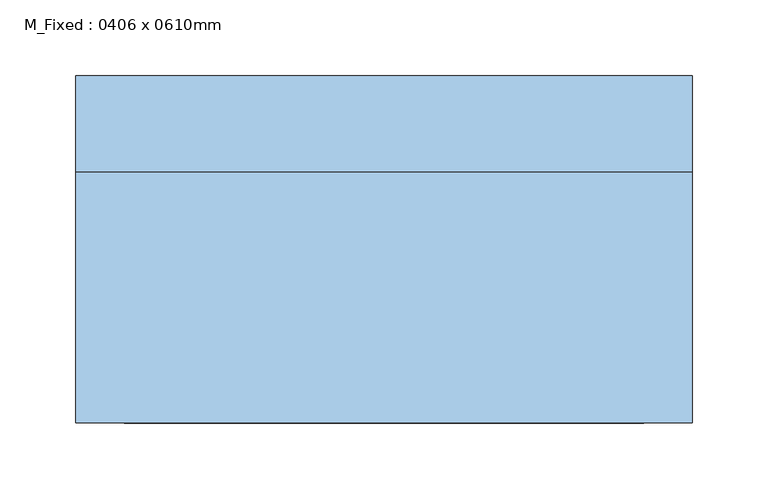
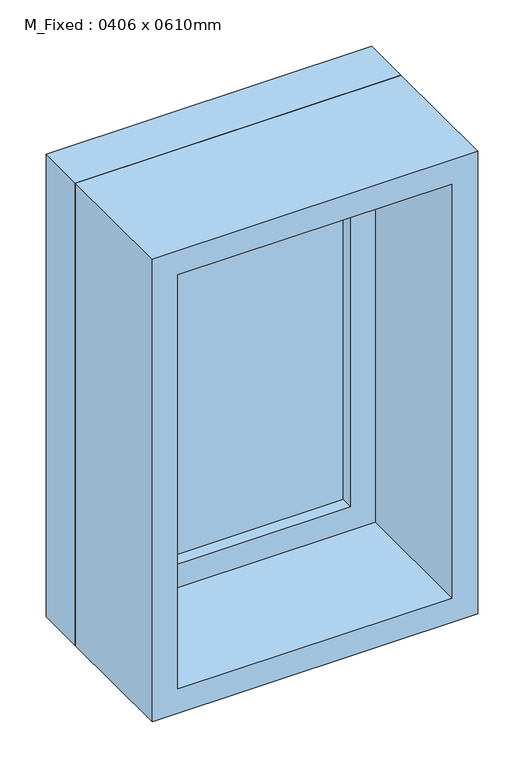
"""IFC4 building model written with IfcOpenShell, lengths in millimetres: window geometry, M_Fixed : 0406 x 0610mm."""

from ifc_helpers import new_model, si_unit, frame, origin, place, context, project, spatial, polyline, outline, extrude, source, transform, mapped, element, save


def m_fixed_0406_x_0610mm_6289636b(model_context):
    return source(origin(), model_context, "Body", "SweptSolid", [
        extrude(outline(polyline([(-140.0, 92.3), (140.0, 92.3), (140.0, 80.3), (-140.0, 80.3), (-140.0, 92.3)])), frame((0.0, 0.0, 978.0), z_axis=(0.0, 0.0, 1.0), x_axis=(1.0, 0.0, 0.0)), (0.0, 0.0, 1.0), 484.0),
        extrude(outline(polyline([(1506.0, -184.0), (934.0, -184.0), (934.0, 184.0), (1506.0, 184.0), (1506.0, -184.0)]), holes=[polyline([(1462.0, -140.0), (1462.0, 140.0), (978.0, 140.0), (978.0, -140.0), (1462.0, -140.0)])]), frame((0.0, 64.3, 0.0), z_axis=(0.0, 1.0, 0.0), x_axis=(0.0, 0.0, 1.0)), (0.0, 0.0, 1.0), 44.0),
        extrude(outline(polyline([(1525.0, -203.0), (915.0, -203.0), (915.0, 203.0), (1525.0, 203.0), (1525.0, -203.0)]), holes=[polyline([(1506.0, -184.0), (1506.0, 184.0), (934.0, 184.0), (934.0, -184.0), (1506.0, -184.0)])]), frame((0.0, 64.3, 0.0), z_axis=(0.0, 1.0, 0.0), x_axis=(0.0, 0.0, 1.0)), (0.0, 0.0, 1.0), 63.0),
        extrude(outline(polyline([(1525.0, -203.0), (915.0, -203.0), (915.0, 203.0), (1525.0, 203.0), (1525.0, -203.0)]), holes=[polyline([(1493.0, -171.0), (1493.0, 171.0), (947.0, 171.0), (947.0, -171.0), (1493.0, -171.0)])]), frame((0.0, -101.3, 0.0), z_axis=(0.0, 1.0, 0.0), x_axis=(0.0, 0.0, 1.0)), (0.0, 0.0, 1.0), 165.6),
    ])


if __name__ == "__main__":
    model = new_model("IFC4")
    model_context = context("Model", 3, world=origin())
    ifc_project = project(units=[si_unit("LENGTHUNIT", "METRE", prefix="MILLI")], contexts=[model_context])
    site = spatial("IfcSite", under=ifc_project)
    building = spatial("IfcBuilding", under=site)
    placement = place(None, origin())
    m_fixed_0406_x_0610mm_shape = m_fixed_0406_x_0610mm_6289636b(model_context)
    element("IfcWindow", 1, ObjectType="M_Fixed : 0406 x 0610mm", at=placement, inside=building, context=model_context, shape_type="MappedRepresentation", body=[
        mapped(m_fixed_0406_x_0610mm_shape, transform((0.0, 0.0, 0.0), x_axis=(1.0, 0.0, 0.0), y_axis=(0.0, 1.0, 0.0), z_axis=(0.0, 0.0, 1.0))),
    ])
    save(model, "model.ifc")

# Revit data of these elements
# Type "M_Fixed : 0406 x 0610mm"
#   Type Mark = "10"
#   Height = 610 mm
#   Default Sill Height = 915 mm
#   Width = 406 mm
#   Window Inset = 19 mm
#   Frame Exterior Material = Sash
#   Frame Interior Material = Sash
#   Glass Pane Material = Glass
#   Sash = Sash
#   Wall Closure = (empty or 0)
# Element 1 (IfcWindow, "M_Fixed : 0406 x 0610mm")
#   Materials on its faces: "Sash", "Glass"
# Materials
#   "Sash": class "Wood", colour RGB 136 99 55, transparency 0
#   "Glass": class "Glass", colour RGB 218 227 224, transparency 0.85, Description = "Soda Lime Glass", Cost = 0
